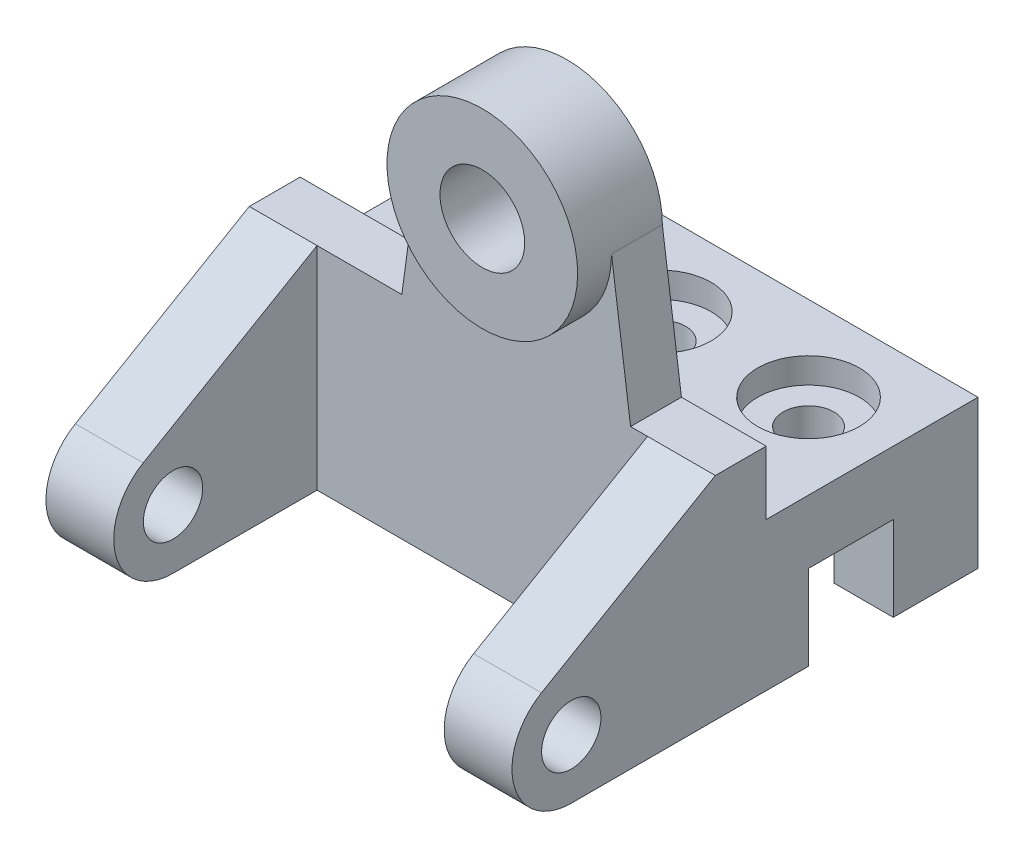
ISO-10303-21;
HEADER;
FILE_DESCRIPTION(('STEP AP214'),'2;1');
FILE_NAME('part.step','',(''),(''),'','','');
FILE_SCHEMA(('AUTOMOTIVE_DESIGN { 1 0 10303 214 1 1 1 1 }'));
ENDSEC;
DATA;
#1=APPLICATION_CONTEXT('core data for automotive mechanical design processes');
#2=APPLICATION_PROTOCOL_DEFINITION('international standard','automotive_design',2000,#1);
#3=PRODUCT_CONTEXT('',#1,'mechanical');
#4=PRODUCT('Part','Part','',(#3));
#5=PRODUCT_RELATED_PRODUCT_CATEGORY('part','',(#4));
#6=PRODUCT_DEFINITION_FORMATION('','',#4);
#7=PRODUCT_DEFINITION_CONTEXT('part definition',#1,'design');
#8=PRODUCT_DEFINITION('design','',#6,#7);
#9=PRODUCT_DEFINITION_SHAPE('','',#8);
#10=(LENGTH_UNIT() NAMED_UNIT(*) SI_UNIT(.MILLI.,.METRE.));
#11=(NAMED_UNIT(*) PLANE_ANGLE_UNIT() SI_UNIT($,.RADIAN.));
#12=(NAMED_UNIT(*) SI_UNIT($,.STERADIAN.) SOLID_ANGLE_UNIT());
#13=UNCERTAINTY_MEASURE_WITH_UNIT(LENGTH_MEASURE(1.E-05),#10,'distance_accuracy_value','');
#14=(GEOMETRIC_REPRESENTATION_CONTEXT(3) GLOBAL_UNCERTAINTY_ASSIGNED_CONTEXT((#13)) GLOBAL_UNIT_ASSIGNED_CONTEXT((#10,
#11,#12)) REPRESENTATION_CONTEXT('',''));
#15=CARTESIAN_POINT('',(0.,0.,0.));
#16=DIRECTION('',(0.,0.,1.));
#17=DIRECTION('',(1.,0.,0.));
#18=AXIS2_PLACEMENT_3D('',#15,#16,#17);
#19=CARTESIAN_POINT('',(-16.,0.,20.));
#20=DIRECTION('',(0.,0.,1.));
#21=DIRECTION('',(1.,0.,0.));
#22=AXIS2_PLACEMENT_3D('',#19,#20,#21);
#23=PLANE('',#22);
#24=DIRECTION('',(0.,1.,0.));
#25=VECTOR('',#24,1.);
#26=CARTESIAN_POINT('',(-14.,-28.999999999873,20.));
#27=LINE('',#26,#25);
#28=CARTESIAN_POINT('',(-14.,0.,20.));
#29=VERTEX_POINT('',#28);
#30=CARTESIAN_POINT('',(-14.,20.,20.));
#31=VERTEX_POINT('',#30);
#32=EDGE_CURVE('E54',#29,#31,#27,.T.);
#33=ORIENTED_EDGE('',*,*,#32,.F.);
#34=DIRECTION('',(1.,0.,0.));
#35=VECTOR('',#34,1.);
#36=CARTESIAN_POINT('',(-16.,0.,20.));
#37=LINE('',#36,#35);
#38=CARTESIAN_POINT('',(0.,0.,20.));
#39=VERTEX_POINT('',#38);
#40=EDGE_CURVE('E235',#29,#39,#37,.T.);
#41=ORIENTED_EDGE('',*,*,#40,.T.);
#42=DIRECTION('',(0.,-1.,0.));
#43=VECTOR('',#42,1.);
#44=CARTESIAN_POINT('',(0.,0.,20.));
#45=LINE('',#44,#43);
#46=CARTESIAN_POINT('',(0.,20.,20.));
#47=VERTEX_POINT('',#46);
#48=EDGE_CURVE('E443',#47,#39,#45,.T.);
#49=ORIENTED_EDGE('',*,*,#48,.F.);
#50=DIRECTION('',(1.,0.,0.));
#51=VECTOR('',#50,1.);
#52=CARTESIAN_POINT('',(-16.,20.,20.));
#53=LINE('',#52,#51);
#54=EDGE_CURVE('E237',#31,#47,#53,.T.);
#55=ORIENTED_EDGE('',*,*,#54,.F.);
#56=EDGE_LOOP('',(#33,#41,#49,#55));
#57=FACE_BOUND('',#56,.T.);
#58=ADVANCED_FACE('F41',(#57),#23,.T.);
#59=DIRECTION('',(0.,1.,0.));
#60=VECTOR('',#59,1.);
#61=CARTESIAN_POINT('',(-26.,-28.999999999873,20.));
#62=LINE('',#61,#60);
#63=CARTESIAN_POINT('',(-26.,20.,20.));
#64=VERTEX_POINT('',#63);
#65=CARTESIAN_POINT('',(-26.,0.,20.));
#66=VERTEX_POINT('',#65);
#67=EDGE_CURVE('E287',#64,#66,#62,.F.);
#68=ORIENTED_EDGE('',*,*,#67,.F.);
#69=CARTESIAN_POINT('',(-49.,20.,20.));
#70=VERTEX_POINT('',#69);
#71=EDGE_CURVE('E239',#70,#64,#53,.T.);
#72=ORIENTED_EDGE('',*,*,#71,.F.);
#73=DIRECTION('',(0.,1.,0.));
#74=VECTOR('',#73,1.);
#75=CARTESIAN_POINT('',(-49.,-28.999999999873,20.));
#76=LINE('',#75,#74);
#77=CARTESIAN_POINT('',(-49.,0.,20.));
#78=VERTEX_POINT('',#77);
#79=EDGE_CURVE('E61',#78,#70,#76,.T.);
#80=ORIENTED_EDGE('',*,*,#79,.F.);
#81=EDGE_CURVE('E240',#78,#66,#37,.T.);
#82=ORIENTED_EDGE('',*,*,#81,.T.);
#83=EDGE_LOOP('',(#68,#72,#80,#82));
#84=FACE_BOUND('',#83,.T.);
#85=ADVANCED_FACE('F453',(#84),#23,.T.);
#86=DIRECTION('',(0.,1.,0.));
#87=VECTOR('',#86,1.);
#88=CARTESIAN_POINT('',(-61.,-28.999999999873,20.));
#89=LINE('',#88,#87);
#90=CARTESIAN_POINT('',(-61.,20.,20.));
#91=VERTEX_POINT('',#90);
#92=CARTESIAN_POINT('',(-61.,0.,20.));
#93=VERTEX_POINT('',#92);
#94=EDGE_CURVE('E273',#91,#93,#89,.F.);
#95=ORIENTED_EDGE('',*,*,#94,.F.);
#96=CARTESIAN_POINT('',(-84.,20.,20.));
#97=VERTEX_POINT('',#96);
#98=EDGE_CURVE('E233',#97,#91,#53,.T.);
#99=ORIENTED_EDGE('',*,*,#98,.F.);
#100=DIRECTION('',(0.,1.,0.));
#101=VECTOR('',#100,1.);
#102=CARTESIAN_POINT('',(-84.,-28.999999999873,20.));
#103=LINE('',#102,#101);
#104=CARTESIAN_POINT('',(-84.,0.,20.));
#105=VERTEX_POINT('',#104);
#106=EDGE_CURVE('E213',#105,#97,#103,.T.);
#107=ORIENTED_EDGE('',*,*,#106,.F.);
#108=EDGE_CURVE('E283',#105,#93,#37,.T.);
#109=ORIENTED_EDGE('',*,*,#108,.T.);
#110=EDGE_LOOP('',(#95,#99,#107,#109));
#111=FACE_BOUND('',#110,.T.);
#112=ADVANCED_FACE('F276',(#111),#23,.T.);
#113=CARTESIAN_POINT('',(-16.,50.000000000127,50.000000000074));
#114=DIRECTION('',(0.,1.,0.));
#115=DIRECTION('',(0.,0.,1.));
#116=AXIS2_PLACEMENT_3D('',#113,#114,#115);
#117=PLANE('',#116);
#118=DIRECTION('',(1.,0.,0.));
#119=VECTOR('',#118,1.);
#120=CARTESIAN_POINT('',(-16.,50.000000000127,50.000000000074));
#121=LINE('',#120,#119);
#122=CARTESIAN_POINT('',(-20.,50.000000000127,50.000000000074));
#123=VERTEX_POINT('',#122);
#124=CARTESIAN_POINT('',(0.,50.000000000127,50.000000000074));
#125=VERTEX_POINT('',#124);
#126=EDGE_CURVE('E261',#123,#125,#121,.T.);
#127=ORIENTED_EDGE('',*,*,#126,.F.);
#128=DIRECTION('',(0.,0.,1.));
#129=VECTOR('',#128,1.);
#130=CARTESIAN_POINT('',(-20.,50.000000000127,50.000000000074));
#131=LINE('',#130,#129);
#132=CARTESIAN_POINT('',(-20.,50.000000000127,62.000000000074));
#133=VERTEX_POINT('',#132);
#134=EDGE_CURVE('E332',#123,#133,#131,.T.);
#135=ORIENTED_EDGE('',*,*,#134,.T.);
#136=DIRECTION('',(1.,0.,0.));
#137=VECTOR('',#136,1.);
#138=CARTESIAN_POINT('',(-110.,50.000000000127,62.000000000074));
#139=LINE('',#138,#137);
#140=CARTESIAN_POINT('',(-16.,50.000000000127,62.000000000074));
#141=VERTEX_POINT('',#140);
#142=EDGE_CURVE('E397',#133,#141,#139,.T.);
#143=ORIENTED_EDGE('',*,*,#142,.T.);
#144=DIRECTION('',(1.,0.,0.));
#145=VECTOR('',#144,1.);
#146=CARTESIAN_POINT('',(-16.,50.000000000127,62.000000000074));
#147=LINE('',#146,#145);
#148=CARTESIAN_POINT('',(0.,50.000000000127,62.000000000074));
#149=VERTEX_POINT('',#148);
#150=EDGE_CURVE('E258',#141,#149,#147,.T.);
#151=ORIENTED_EDGE('',*,*,#150,.T.);
#152=DIRECTION('',(0.,0.,1.));
#153=VECTOR('',#152,1.);
#154=CARTESIAN_POINT('',(0.,50.000000000127,50.000000000074));
#155=LINE('',#154,#153);
#156=EDGE_CURVE('E430',#125,#149,#155,.T.);
#157=ORIENTED_EDGE('',*,*,#156,.F.);
#158=EDGE_LOOP('',(#127,#135,#143,#151,#157));
#159=FACE_BOUND('',#158,.T.);
#160=ADVANCED_FACE('F559',(#159),#117,.T.);
#161=CARTESIAN_POINT('',(-110.,50.000000000127,62.000000000074));
#162=DIRECTION('',(0.,0.,-1.));
#163=DIRECTION('',(-1.,0.,0.));
#164=AXIS2_PLACEMENT_3D('',#161,#162,#163);
#165=PLANE('',#164);
#166=DIRECTION('',(0.,-1.,0.));
#167=VECTOR('',#166,1.);
#168=CARTESIAN_POINT('',(-94.,0.,62.000000000074));
#169=LINE('',#168,#167);
#170=CARTESIAN_POINT('',(-94.,50.000000000127,62.000000000074));
#171=VERTEX_POINT('',#170);
#172=CARTESIAN_POINT('',(-94.,0.,62.000000000074));
#173=VERTEX_POINT('',#172);
#174=EDGE_CURVE('E364',#171,#173,#169,.T.);
#175=ORIENTED_EDGE('',*,*,#174,.T.);
#176=DIRECTION('',(1.,0.,0.));
#177=VECTOR('',#176,1.);
#178=CARTESIAN_POINT('',(-110.,0.,62.000000000074));
#179=LINE('',#178,#177);
#180=CARTESIAN_POINT('',(-16.,0.,62.000000000074));
#181=VERTEX_POINT('',#180);
#182=EDGE_CURVE('E408',#173,#181,#179,.T.);
#183=ORIENTED_EDGE('',*,*,#182,.T.);
#184=DIRECTION('',(0.,1.,0.));
#185=VECTOR('',#184,1.);
#186=CARTESIAN_POINT('',(-16.,50.000000000127,62.000000000074));
#187=LINE('',#186,#185);
#188=EDGE_CURVE('E372',#181,#141,#187,.T.);
#189=ORIENTED_EDGE('',*,*,#188,.T.);
#190=ORIENTED_EDGE('',*,*,#142,.F.);
#191=DIRECTION('',(-0.135113204733824,0.990830168044229,0.));
#192=VECTOR('',#191,1.);
#193=CARTESIAN_POINT('',(-20.,50.000000000127,62.000000000074));
#194=LINE('',#193,#192);
#195=CARTESIAN_POINT('',(-24.5,83.,62.000000000074));
#196=VERTEX_POINT('',#195);
#197=EDGE_CURVE('E322',#133,#196,#194,.T.);
#198=ORIENTED_EDGE('',*,*,#197,.T.);
#199=CARTESIAN_POINT('',(-47.,83.,62.000000000074));
#200=DIRECTION('',(0.,0.,-1.));
#201=DIRECTION('',(1.,0.,0.));
#202=AXIS2_PLACEMENT_3D('',#199,#200,#201);
#203=CIRCLE('',#202,22.5);
#204=CARTESIAN_POINT('',(-69.5,83.,62.000000000074));
#205=VERTEX_POINT('',#204);
#206=EDGE_CURVE('E331',#196,#205,#203,.T.);
#207=ORIENTED_EDGE('',*,*,#206,.T.);
#208=DIRECTION('',(-0.135113204733824,-0.990830168044229,0.));
#209=VECTOR('',#208,1.);
#210=CARTESIAN_POINT('',(-74.,50.000000000127,62.000000000074));
#211=LINE('',#210,#209);
#212=CARTESIAN_POINT('',(-74.,50.000000000127,62.000000000074));
#213=VERTEX_POINT('',#212);
#214=EDGE_CURVE('E328',#205,#213,#211,.T.);
#215=ORIENTED_EDGE('',*,*,#214,.T.);
#216=EDGE_CURVE('E410',#171,#213,#139,.T.);
#217=ORIENTED_EDGE('',*,*,#216,.F.);
#218=EDGE_LOOP('',(#175,#183,#189,#190,#198,#207,#215,#217));
#219=FACE_BOUND('',#218,.T.);
#220=ADVANCED_FACE('F563',(#219),#165,.F.);
#221=CARTESIAN_POINT('',(-16.,14.,96.));
#222=DIRECTION('',(1.,0.,0.));
#223=DIRECTION('',(0.,0.,-1.));
#224=AXIS2_PLACEMENT_3D('',#221,#222,#223);
#225=PLANE('',#224);
#226=CARTESIAN_POINT('',(-16.,14.,96.));
#227=DIRECTION('',(1.,0.,0.));
#228=DIRECTION('',(0.,0.,-1.));
#229=AXIS2_PLACEMENT_3D('',#226,#227,#228);
#230=CIRCLE('',#229,7.);
#231=CARTESIAN_POINT('',(-16.,14.,89.));
#232=VERTEX_POINT('',#231);
#233=EDGE_CURVE('E355',#232,#232,#230,.T.);
#234=ORIENTED_EDGE('',*,*,#233,.T.);
#235=EDGE_LOOP('',(#234));
#236=FACE_BOUND('',#235,.T.);
#237=ORIENTED_EDGE('',*,*,#188,.F.);
#238=DIRECTION('',(0.,0.,-1.));
#239=VECTOR('',#238,1.);
#240=CARTESIAN_POINT('',(-16.,0.,40.));
#241=LINE('',#240,#239);
#242=CARTESIAN_POINT('',(-16.,0.,96.));
#243=VERTEX_POINT('',#242);
#244=EDGE_CURVE('E266',#243,#181,#241,.T.);
#245=ORIENTED_EDGE('',*,*,#244,.F.);
#246=CARTESIAN_POINT('',(-16.,14.,96.));
#247=DIRECTION('',(1.,0.,0.));
#248=DIRECTION('',(0.,0.,-1.));
#249=AXIS2_PLACEMENT_3D('',#246,#247,#248);
#250=CIRCLE('',#249,14.);
#251=CARTESIAN_POINT('',(-16.,26.0981840675639,103.045136071599));
#252=VERTEX_POINT('',#251);
#253=EDGE_CURVE('E415',#252,#243,#250,.T.);
#254=ORIENTED_EDGE('',*,*,#253,.F.);
#255=DIRECTION('',(0.,-0.5032240051142,0.864156004825994));
#256=VECTOR('',#255,1.);
#257=CARTESIAN_POINT('',(-16.,50.000000000127,62.000000000074));
#258=LINE('',#257,#256);
#259=EDGE_CURVE('E409',#141,#252,#258,.T.);
#260=ORIENTED_EDGE('',*,*,#259,.F.);
#261=EDGE_LOOP('',(#237,#245,#254,#260));
#262=FACE_BOUND('',#261,.T.);
#263=ADVANCED_FACE('F573',(#236,#262),#225,.F.);
#264=CARTESIAN_POINT('',(-16.,0.,0.));
#265=DIRECTION('',(0.,0.,-1.));
#266=DIRECTION('',(0.,1.,0.));
#267=AXIS2_PLACEMENT_3D('',#264,#265,#266);
#268=PLANE('',#267);
#269=DIRECTION('',(0.,1.,0.));
#270=VECTOR('',#269,1.);
#271=CARTESIAN_POINT('',(0.,0.,0.));
#272=LINE('',#271,#270);
#273=CARTESIAN_POINT('',(0.,0.,0.));
#274=VERTEX_POINT('',#273);
#275=CARTESIAN_POINT('',(0.,35.0000000001271,0.));
#276=VERTEX_POINT('',#275);
#277=EDGE_CURVE('E407',#274,#276,#272,.T.);
#278=ORIENTED_EDGE('',*,*,#277,.F.);
#279=DIRECTION('',(1.,0.,0.));
#280=VECTOR('',#279,1.);
#281=CARTESIAN_POINT('',(-16.,0.,0.));
#282=LINE('',#281,#280);
#283=CARTESIAN_POINT('',(-110.,0.,0.));
#284=VERTEX_POINT('',#283);
#285=EDGE_CURVE('E217',#284,#274,#282,.T.);
#286=ORIENTED_EDGE('',*,*,#285,.F.);
#287=DIRECTION('',(0.,-1.,0.));
#288=VECTOR('',#287,1.);
#289=CARTESIAN_POINT('',(-110.,0.,0.));
#290=LINE('',#289,#288);
#291=CARTESIAN_POINT('',(-110.,35.0000000001271,0.));
#292=VERTEX_POINT('',#291);
#293=EDGE_CURVE('E396',#292,#284,#290,.T.);
#294=ORIENTED_EDGE('',*,*,#293,.F.);
#295=DIRECTION('',(1.,0.,0.));
#296=VECTOR('',#295,1.);
#297=CARTESIAN_POINT('',(-16.,35.0000000001271,0.));
#298=LINE('',#297,#296);
#299=EDGE_CURVE('E262',#292,#276,#298,.T.);
#300=ORIENTED_EDGE('',*,*,#299,.T.);
#301=EDGE_LOOP('',(#278,#286,#294,#300));
#302=FACE_BOUND('',#301,.T.);
#303=ADVANCED_FACE('F43',(#302),#268,.T.);
#304=CARTESIAN_POINT('',(-16.,0.,0.));
#305=DIRECTION('',(0.,-1.,0.));
#306=DIRECTION('',(0.,0.,-1.));
#307=AXIS2_PLACEMENT_3D('',#304,#305,#306);
#308=PLANE('',#307);
#309=CARTESIAN_POINT('',(-20.,0.,20.000000000074));
#310=DIRECTION('',(0.,-1.,0.));
#311=DIRECTION('',(0.,0.,-1.));
#312=AXIS2_PLACEMENT_3D('',#309,#310,#311);
#313=CIRCLE('',#312,6.);
#314=EDGE_CURVE('E291',#66,#29,#313,.T.);
#315=ORIENTED_EDGE('',*,*,#314,.F.);
#316=ORIENTED_EDGE('',*,*,#81,.F.);
#317=CARTESIAN_POINT('',(-55.,0.,20.000000000074));
#318=DIRECTION('',(0.,-1.,0.));
#319=DIRECTION('',(0.,0.,-1.));
#320=AXIS2_PLACEMENT_3D('',#317,#318,#319);
#321=CIRCLE('',#320,6.);
#322=EDGE_CURVE('E282',#93,#78,#321,.T.);
#323=ORIENTED_EDGE('',*,*,#322,.F.);
#324=ORIENTED_EDGE('',*,*,#108,.F.);
#325=CARTESIAN_POINT('',(-90.,0.,20.000000000074));
#326=DIRECTION('',(0.,-1.,0.));
#327=DIRECTION('',(0.,0.,-1.));
#328=AXIS2_PLACEMENT_3D('',#325,#326,#327);
#329=CIRCLE('',#328,6.);
#330=CARTESIAN_POINT('',(-96.,0.,20.));
#331=VERTEX_POINT('',#330);
#332=EDGE_CURVE('E285',#331,#105,#329,.T.);
#333=ORIENTED_EDGE('',*,*,#332,.F.);
#334=CARTESIAN_POINT('',(-110.,0.,20.));
#335=VERTEX_POINT('',#334);
#336=EDGE_CURVE('E228',#335,#331,#37,.T.);
#337=ORIENTED_EDGE('',*,*,#336,.F.);
#338=DIRECTION('',(0.,0.,1.));
#339=VECTOR('',#338,1.);
#340=CARTESIAN_POINT('',(-110.,0.,20.));
#341=LINE('',#340,#339);
#342=EDGE_CURVE('E380',#284,#335,#341,.T.);
#343=ORIENTED_EDGE('',*,*,#342,.F.);
#344=ORIENTED_EDGE('',*,*,#285,.T.);
#345=DIRECTION('',(0.,0.,-1.));
#346=VECTOR('',#345,1.);
#347=CARTESIAN_POINT('',(0.,0.,0.));
#348=LINE('',#347,#346);
#349=EDGE_CURVE('E413',#39,#274,#348,.T.);
#350=ORIENTED_EDGE('',*,*,#349,.F.);
#351=ORIENTED_EDGE('',*,*,#40,.F.);
#352=EDGE_LOOP('',(#315,#316,#323,#324,#333,#337,#343,#344,#350,#351));
#353=FACE_BOUND('',#352,.T.);
#354=ADVANCED_FACE('F460',(#353),#308,.T.);
#355=DIRECTION('',(0.,1.,0.));
#356=VECTOR('',#355,1.);
#357=CARTESIAN_POINT('',(-96.,-28.999999999873,20.));
#358=LINE('',#357,#356);
#359=CARTESIAN_POINT('',(-96.,20.,20.));
#360=VERTEX_POINT('',#359);
#361=EDGE_CURVE('E209',#360,#331,#358,.F.);
#362=ORIENTED_EDGE('',*,*,#361,.F.);
#363=CARTESIAN_POINT('',(-110.,20.,20.));
#364=VERTEX_POINT('',#363);
#365=EDGE_CURVE('E221',#364,#360,#53,.T.);
#366=ORIENTED_EDGE('',*,*,#365,.F.);
#367=DIRECTION('',(0.,1.,0.));
#368=VECTOR('',#367,1.);
#369=CARTESIAN_POINT('',(-110.,20.,20.));
#370=LINE('',#369,#368);
#371=EDGE_CURVE('E379',#335,#364,#370,.T.);
#372=ORIENTED_EDGE('',*,*,#371,.F.);
#373=ORIENTED_EDGE('',*,*,#336,.T.);
#374=EDGE_LOOP('',(#362,#366,#372,#373));
#375=FACE_BOUND('',#374,.T.);
#376=ADVANCED_FACE('F225',(#375),#23,.T.);
#377=CARTESIAN_POINT('',(-16.,20.,20.));
#378=DIRECTION('',(0.,-1.,0.));
#379=DIRECTION('',(0.,0.,-1.));
#380=AXIS2_PLACEMENT_3D('',#377,#378,#379);
#381=PLANE('',#380);
#382=CARTESIAN_POINT('',(-20.,20.,20.000000000074));
#383=DIRECTION('',(0.,-1.,0.));
#384=DIRECTION('',(0.,0.,-1.));
#385=AXIS2_PLACEMENT_3D('',#382,#383,#384);
#386=CIRCLE('',#385,6.);
#387=EDGE_CURVE('E11',#31,#64,#386,.T.);
#388=ORIENTED_EDGE('',*,*,#387,.F.);
#389=ORIENTED_EDGE('',*,*,#54,.T.);
#390=DIRECTION('',(0.,0.,-1.));
#391=VECTOR('',#390,1.);
#392=CARTESIAN_POINT('',(0.,20.,20.));
#393=LINE('',#392,#391);
#394=CARTESIAN_POINT('',(0.,20.,40.));
#395=VERTEX_POINT('',#394);
#396=EDGE_CURVE('E445',#395,#47,#393,.T.);
#397=ORIENTED_EDGE('',*,*,#396,.F.);
#398=DIRECTION('',(1.,0.,0.));
#399=VECTOR('',#398,1.);
#400=CARTESIAN_POINT('',(-16.,20.,40.));
#401=LINE('',#400,#399);
#402=CARTESIAN_POINT('',(-110.,20.,40.));
#403=VERTEX_POINT('',#402);
#404=EDGE_CURVE('E243',#403,#395,#401,.T.);
#405=ORIENTED_EDGE('',*,*,#404,.F.);
#406=DIRECTION('',(0.,0.,1.));
#407=VECTOR('',#406,1.);
#408=CARTESIAN_POINT('',(-110.,20.,40.));
#409=LINE('',#408,#407);
#410=EDGE_CURVE('E231',#364,#403,#409,.T.);
#411=ORIENTED_EDGE('',*,*,#410,.F.);
#412=ORIENTED_EDGE('',*,*,#365,.T.);
#413=CARTESIAN_POINT('',(-90.,20.,20.000000000074));
#414=DIRECTION('',(0.,-1.,0.));
#415=DIRECTION('',(0.,0.,-1.));
#416=AXIS2_PLACEMENT_3D('',#413,#414,#415);
#417=CIRCLE('',#416,6.);
#418=EDGE_CURVE('E206',#97,#360,#417,.T.);
#419=ORIENTED_EDGE('',*,*,#418,.F.);
#420=ORIENTED_EDGE('',*,*,#98,.T.);
#421=CARTESIAN_POINT('',(-55.,20.,20.000000000074));
#422=DIRECTION('',(0.,-1.,0.));
#423=DIRECTION('',(0.,0.,-1.));
#424=AXIS2_PLACEMENT_3D('',#421,#422,#423);
#425=CIRCLE('',#424,6.);
#426=EDGE_CURVE('E47',#70,#91,#425,.T.);
#427=ORIENTED_EDGE('',*,*,#426,.F.);
#428=ORIENTED_EDGE('',*,*,#71,.T.);
#429=EDGE_LOOP('',(#388,#389,#397,#405,#411,#412,#419,#420,#427,#428));
#430=FACE_BOUND('',#429,.T.);
#431=ADVANCED_FACE('F229',(#430),#381,.T.);
#432=CARTESIAN_POINT('',(-16.,20.,40.));
#433=DIRECTION('',(0.,0.,-1.));
#434=DIRECTION('',(-1.,0.,0.));
#435=AXIS2_PLACEMENT_3D('',#432,#433,#434);
#436=PLANE('',#435);
#437=DIRECTION('',(0.,1.,0.));
#438=VECTOR('',#437,1.);
#439=CARTESIAN_POINT('',(0.,20.,40.));
#440=LINE('',#439,#438);
#441=CARTESIAN_POINT('',(0.,0.,40.));
#442=VERTEX_POINT('',#441);
#443=EDGE_CURVE('E438',#442,#395,#440,.T.);
#444=ORIENTED_EDGE('',*,*,#443,.F.);
#445=DIRECTION('',(1.,0.,0.));
#446=VECTOR('',#445,1.);
#447=CARTESIAN_POINT('',(-16.,0.,40.));
#448=LINE('',#447,#446);
#449=CARTESIAN_POINT('',(-110.,0.,40.));
#450=VERTEX_POINT('',#449);
#451=EDGE_CURVE('E249',#450,#442,#448,.T.);
#452=ORIENTED_EDGE('',*,*,#451,.F.);
#453=DIRECTION('',(0.,-1.,0.));
#454=VECTOR('',#453,1.);
#455=CARTESIAN_POINT('',(-110.,0.,40.));
#456=LINE('',#455,#454);
#457=EDGE_CURVE('E382',#403,#450,#456,.T.);
#458=ORIENTED_EDGE('',*,*,#457,.F.);
#459=ORIENTED_EDGE('',*,*,#404,.T.);
#460=EDGE_LOOP('',(#444,#452,#458,#459));
#461=FACE_BOUND('',#460,.T.);
#462=ADVANCED_FACE('F470',(#461),#436,.T.);
#463=CARTESIAN_POINT('',(-16.,0.,40.));
#464=DIRECTION('',(0.,-1.,0.));
#465=DIRECTION('',(0.,0.,-1.));
#466=AXIS2_PLACEMENT_3D('',#463,#464,#465);
#467=PLANE('',#466);
#468=DIRECTION('',(0.,0.,-1.));
#469=VECTOR('',#468,1.);
#470=CARTESIAN_POINT('',(0.,0.,40.));
#471=LINE('',#470,#469);
#472=CARTESIAN_POINT('',(0.,0.,96.));
#473=VERTEX_POINT('',#472);
#474=EDGE_CURVE('E436',#473,#442,#471,.T.);
#475=ORIENTED_EDGE('',*,*,#474,.F.);
#476=DIRECTION('',(1.,0.,0.));
#477=VECTOR('',#476,1.);
#478=CARTESIAN_POINT('',(-16.,0.,96.));
#479=LINE('',#478,#477);
#480=EDGE_CURVE('E247',#243,#473,#479,.T.);
#481=ORIENTED_EDGE('',*,*,#480,.F.);
#482=ORIENTED_EDGE('',*,*,#244,.T.);
#483=ORIENTED_EDGE('',*,*,#182,.F.);
#484=DIRECTION('',(0.,0.,1.));
#485=VECTOR('',#484,1.);
#486=CARTESIAN_POINT('',(-94.,0.,62.000000000074));
#487=LINE('',#486,#485);
#488=CARTESIAN_POINT('',(-94.,0.,96.0000000000002));
#489=VERTEX_POINT('',#488);
#490=EDGE_CURVE('E359',#173,#489,#487,.T.);
#491=ORIENTED_EDGE('',*,*,#490,.T.);
#492=DIRECTION('',(-1.,0.,0.));
#493=VECTOR('',#492,1.);
#494=CARTESIAN_POINT('',(-94.,0.,96.0000000000002));
#495=LINE('',#494,#493);
#496=CARTESIAN_POINT('',(-110.,0.,96.0000000000002));
#497=VERTEX_POINT('',#496);
#498=EDGE_CURVE('E366',#489,#497,#495,.T.);
#499=ORIENTED_EDGE('',*,*,#498,.T.);
#500=DIRECTION('',(0.,0.,1.));
#501=VECTOR('',#500,1.);
#502=CARTESIAN_POINT('',(-110.,0.,62.000000000074));
#503=LINE('',#502,#501);
#504=EDGE_CURVE('E387',#450,#497,#503,.T.);
#505=ORIENTED_EDGE('',*,*,#504,.F.);
#506=ORIENTED_EDGE('',*,*,#451,.T.);
#507=EDGE_LOOP('',(#475,#481,#482,#483,#491,#499,#505,#506));
#508=FACE_BOUND('',#507,.T.);
#509=ADVANCED_FACE('F473',(#508),#467,.T.);
#510=CARTESIAN_POINT('',(-16.,14.,96.));
#511=DIRECTION('',(1.,0.,0.));
#512=DIRECTION('',(0.,0.,-1.));
#513=AXIS2_PLACEMENT_3D('',#510,#511,#512);
#514=CYLINDRICAL_SURFACE('',#513,14.);
#515=CARTESIAN_POINT('',(0.,14.,96.));
#516=DIRECTION('',(1.,0.,0.));
#517=DIRECTION('',(0.,0.,-1.));
#518=AXIS2_PLACEMENT_3D('',#515,#516,#517);
#519=CIRCLE('',#518,14.);
#520=CARTESIAN_POINT('',(0.,26.0981840675639,103.045136071599));
#521=VERTEX_POINT('',#520);
#522=EDGE_CURVE('E433',#521,#473,#519,.T.);
#523=ORIENTED_EDGE('',*,*,#522,.F.);
#524=DIRECTION('',(1.,0.,0.));
#525=VECTOR('',#524,1.);
#526=CARTESIAN_POINT('',(-16.,26.0981840675639,103.045136071599));
#527=LINE('',#526,#525);
#528=EDGE_CURVE('E255',#252,#521,#527,.T.);
#529=ORIENTED_EDGE('',*,*,#528,.F.);
#530=ORIENTED_EDGE('',*,*,#253,.T.);
#531=ORIENTED_EDGE('',*,*,#480,.T.);
#532=EDGE_LOOP('',(#523,#529,#530,#531));
#533=FACE_BOUND('',#532,.T.);
#534=ADVANCED_FACE('F584',(#533),#514,.T.);
#535=CARTESIAN_POINT('',(-16.,50.000000000127,62.000000000074));
#536=DIRECTION('',(0.,0.864156004825994,0.5032240051142));
#537=DIRECTION('',(0.,-0.5032240051142,0.864156004825994));
#538=AXIS2_PLACEMENT_3D('',#535,#536,#537);
#539=PLANE('',#538);
#540=DIRECTION('',(0.,-0.5032240051142,0.864156004825994));
#541=VECTOR('',#540,1.);
#542=CARTESIAN_POINT('',(0.,50.000000000127,62.000000000074));
#543=LINE('',#542,#541);
#544=EDGE_CURVE('E429',#149,#521,#543,.T.);
#545=ORIENTED_EDGE('',*,*,#544,.F.);
#546=ORIENTED_EDGE('',*,*,#150,.F.);
#547=ORIENTED_EDGE('',*,*,#259,.T.);
#548=ORIENTED_EDGE('',*,*,#528,.T.);
#549=EDGE_LOOP('',(#545,#546,#547,#548));
#550=FACE_BOUND('',#549,.T.);
#551=ADVANCED_FACE('F580',(#550),#539,.T.);
#552=DIRECTION('',(0.,0.,1.));
#553=VECTOR('',#552,1.);
#554=CARTESIAN_POINT('',(-74.,50.000000000127,50.000000000074));
#555=LINE('',#554,#553);
#556=CARTESIAN_POINT('',(-74.,50.000000000127,50.000000000074));
#557=VERTEX_POINT('',#556);
#558=EDGE_CURVE('E337',#557,#213,#555,.T.);
#559=ORIENTED_EDGE('',*,*,#558,.F.);
#560=CARTESIAN_POINT('',(-110.,50.000000000127,50.000000000074));
#561=VERTEX_POINT('',#560);
#562=EDGE_CURVE('E256',#561,#557,#121,.T.);
#563=ORIENTED_EDGE('',*,*,#562,.F.);
#564=DIRECTION('',(0.,0.,-1.));
#565=VECTOR('',#564,1.);
#566=CARTESIAN_POINT('',(-110.,50.000000000127,50.000000000074));
#567=LINE('',#566,#565);
#568=CARTESIAN_POINT('',(-110.,50.000000000127,62.000000000074));
#569=VERTEX_POINT('',#568);
#570=EDGE_CURVE('E389',#569,#561,#567,.T.);
#571=ORIENTED_EDGE('',*,*,#570,.F.);
#572=EDGE_CURVE('E401',#569,#171,#139,.T.);
#573=ORIENTED_EDGE('',*,*,#572,.T.);
#574=ORIENTED_EDGE('',*,*,#216,.T.);
#575=EDGE_LOOP('',(#559,#563,#571,#573,#574));
#576=FACE_BOUND('',#575,.T.);
#577=ADVANCED_FACE('F486',(#576),#117,.T.);
#578=CARTESIAN_POINT('',(-16.,35.0000000001271,50.000000000074));
#579=DIRECTION('',(0.,0.,-1.));
#580=DIRECTION('',(0.,1.,0.));
#581=AXIS2_PLACEMENT_3D('',#578,#579,#580);
#582=PLANE('',#581);
#583=CARTESIAN_POINT('',(-47.,83.,50.000000000074));
#584=DIRECTION('',(0.,0.,-1.));
#585=DIRECTION('',(0.,1.,0.));
#586=AXIS2_PLACEMENT_3D('',#583,#584,#585);
#587=CIRCLE('',#586,10.);
#588=CARTESIAN_POINT('',(-47.,93.,50.000000000074));
#589=VERTEX_POINT('',#588);
#590=EDGE_CURVE('E316',#589,#589,#587,.T.);
#591=ORIENTED_EDGE('',*,*,#590,.F.);
#592=EDGE_LOOP('',(#591));
#593=FACE_BOUND('',#592,.T.);
#594=DIRECTION('',(0.,1.,0.));
#595=VECTOR('',#594,1.);
#596=CARTESIAN_POINT('',(0.,35.0000000001271,50.000000000074));
#597=LINE('',#596,#595);
#598=CARTESIAN_POINT('',(0.,35.0000000001271,50.000000000074));
#599=VERTEX_POINT('',#598);
#600=EDGE_CURVE('E424',#599,#125,#597,.T.);
#601=ORIENTED_EDGE('',*,*,#600,.F.);
#602=DIRECTION('',(1.,0.,0.));
#603=VECTOR('',#602,1.);
#604=CARTESIAN_POINT('',(-16.,35.0000000001271,50.000000000074));
#605=LINE('',#604,#603);
#606=CARTESIAN_POINT('',(-110.,35.0000000001271,50.000000000074));
#607=VERTEX_POINT('',#606);
#608=EDGE_CURVE('E265',#607,#599,#605,.T.);
#609=ORIENTED_EDGE('',*,*,#608,.F.);
#610=DIRECTION('',(0.,-1.,0.));
#611=VECTOR('',#610,1.);
#612=CARTESIAN_POINT('',(-110.,35.0000000001271,50.000000000074));
#613=LINE('',#612,#611);
#614=EDGE_CURVE('E393',#561,#607,#613,.T.);
#615=ORIENTED_EDGE('',*,*,#614,.F.);
#616=ORIENTED_EDGE('',*,*,#562,.T.);
#617=DIRECTION('',(-0.135113204733824,-0.990830168044229,0.));
#618=VECTOR('',#617,1.);
#619=CARTESIAN_POINT('',(-74.,50.000000000127,50.000000000074));
#620=LINE('',#619,#618);
#621=CARTESIAN_POINT('',(-69.5,83.,50.000000000074));
#622=VERTEX_POINT('',#621);
#623=EDGE_CURVE('E327',#622,#557,#620,.T.);
#624=ORIENTED_EDGE('',*,*,#623,.F.);
#625=CARTESIAN_POINT('',(-47.,83.,50.000000000074));
#626=DIRECTION('',(0.,0.,1.));
#627=DIRECTION('',(1.,0.,0.));
#628=AXIS2_PLACEMENT_3D('',#625,#626,#627);
#629=CIRCLE('',#628,22.5);
#630=CARTESIAN_POINT('',(-24.5,83.,50.000000000074));
#631=VERTEX_POINT('',#630);
#632=EDGE_CURVE('E325',#631,#622,#629,.T.);
#633=ORIENTED_EDGE('',*,*,#632,.F.);
#634=DIRECTION('',(-0.135113204733824,0.990830168044229,0.));
#635=VECTOR('',#634,1.);
#636=CARTESIAN_POINT('',(-20.,50.000000000127,50.000000000074));
#637=LINE('',#636,#635);
#638=EDGE_CURVE('E324',#123,#631,#637,.T.);
#639=ORIENTED_EDGE('',*,*,#638,.F.);
#640=ORIENTED_EDGE('',*,*,#126,.T.);
#641=EDGE_LOOP('',(#601,#609,#615,#616,#624,#633,#639,#640));
#642=FACE_BOUND('',#641,.T.);
#643=ADVANCED_FACE('F491',(#593,#642),#582,.T.);
#644=CARTESIAN_POINT('',(-16.,35.0000000001271,0.));
#645=DIRECTION('',(0.,1.,0.));
#646=DIRECTION('',(0.,0.,1.));
#647=AXIS2_PLACEMENT_3D('',#644,#645,#646);
#648=PLANE('',#647);
#649=CARTESIAN_POINT('',(-20.,35.0000000001271,20.000000000074));
#650=DIRECTION('',(0.,1.,0.));
#651=DIRECTION('',(0.,0.,1.));
#652=AXIS2_PLACEMENT_3D('',#649,#650,#651);
#653=CIRCLE('',#652,12.);
#654=CARTESIAN_POINT('',(-20.,35.0000000001271,32.000000000074));
#655=VERTEX_POINT('',#654);
#656=EDGE_CURVE('E299',#655,#655,#653,.T.);
#657=ORIENTED_EDGE('',*,*,#656,.F.);
#658=EDGE_LOOP('',(#657));
#659=FACE_BOUND('',#658,.T.);
#660=CARTESIAN_POINT('',(-55.,35.0000000001271,20.000000000074));
#661=DIRECTION('',(0.,1.,0.));
#662=DIRECTION('',(0.,0.,1.));
#663=AXIS2_PLACEMENT_3D('',#660,#661,#662);
#664=CIRCLE('',#663,12.);
#665=CARTESIAN_POINT('',(-55.,35.0000000001271,32.000000000074));
#666=VERTEX_POINT('',#665);
#667=EDGE_CURVE('E308',#666,#666,#664,.T.);
#668=ORIENTED_EDGE('',*,*,#667,.F.);
#669=EDGE_LOOP('',(#668));
#670=FACE_BOUND('',#669,.T.);
#671=CARTESIAN_POINT('',(-90.,35.0000000001271,20.000000000074));
#672=DIRECTION('',(0.,1.,0.));
#673=DIRECTION('',(0.,0.,1.));
#674=AXIS2_PLACEMENT_3D('',#671,#672,#673);
#675=CIRCLE('',#674,12.0000000000216);
#676=CARTESIAN_POINT('',(-90.,35.0000000001271,32.0000000000956));
#677=VERTEX_POINT('',#676);
#678=EDGE_CURVE('E293',#677,#677,#675,.T.);
#679=ORIENTED_EDGE('',*,*,#678,.F.);
#680=EDGE_LOOP('',(#679));
#681=FACE_BOUND('',#680,.T.);
#682=DIRECTION('',(0.,0.,1.));
#683=VECTOR('',#682,1.);
#684=CARTESIAN_POINT('',(0.,35.0000000001271,0.));
#685=LINE('',#684,#683);
#686=EDGE_CURVE('E423',#276,#599,#685,.T.);
#687=ORIENTED_EDGE('',*,*,#686,.F.);
#688=ORIENTED_EDGE('',*,*,#299,.F.);
#689=DIRECTION('',(0.,0.,-1.));
#690=VECTOR('',#689,1.);
#691=CARTESIAN_POINT('',(-110.,35.0000000001271,0.));
#692=LINE('',#691,#690);
#693=EDGE_CURVE('E392',#607,#292,#692,.T.);
#694=ORIENTED_EDGE('',*,*,#693,.F.);
#695=ORIENTED_EDGE('',*,*,#608,.T.);
#696=EDGE_LOOP('',(#687,#688,#694,#695));
#697=FACE_BOUND('',#696,.T.);
#698=ADVANCED_FACE('F494',(#659,#670,#681,#697),#648,.T.);
#699=CARTESIAN_POINT('',(0.,14.,96.));
#700=DIRECTION('',(1.,0.,0.));
#701=DIRECTION('',(0.,0.,-1.));
#702=AXIS2_PLACEMENT_3D('',#699,#700,#701);
#703=PLANE('',#702);
#704=CARTESIAN_POINT('',(0.,14.,96.));
#705=DIRECTION('',(1.,0.,0.));
#706=DIRECTION('',(0.,0.,-1.));
#707=AXIS2_PLACEMENT_3D('',#704,#705,#706);
#708=CIRCLE('',#707,7.);
#709=CARTESIAN_POINT('',(0.,14.,89.));
#710=VERTEX_POINT('',#709);
#711=EDGE_CURVE('E269',#710,#710,#708,.T.);
#712=ORIENTED_EDGE('',*,*,#711,.F.);
#713=EDGE_LOOP('',(#712));
#714=FACE_BOUND('',#713,.T.);
#715=ORIENTED_EDGE('',*,*,#277,.T.);
#716=ORIENTED_EDGE('',*,*,#686,.T.);
#717=ORIENTED_EDGE('',*,*,#600,.T.);
#718=ORIENTED_EDGE('',*,*,#156,.T.);
#719=ORIENTED_EDGE('',*,*,#544,.T.);
#720=ORIENTED_EDGE('',*,*,#522,.T.);
#721=ORIENTED_EDGE('',*,*,#474,.T.);
#722=ORIENTED_EDGE('',*,*,#443,.T.);
#723=ORIENTED_EDGE('',*,*,#396,.T.);
#724=ORIENTED_EDGE('',*,*,#48,.T.);
#725=ORIENTED_EDGE('',*,*,#349,.T.);
#726=EDGE_LOOP('',(#715,#716,#717,#718,#719,#720,#721,#722,#723,#724,#725));
#727=FACE_BOUND('',#726,.T.);
#728=ADVANCED_FACE('F462',(#714,#727),#703,.T.);
#729=CARTESIAN_POINT('',(-110.,0.,0.));
#730=DIRECTION('',(1.,0.,0.));
#731=DIRECTION('',(0.,0.,-1.));
#732=AXIS2_PLACEMENT_3D('',#729,#730,#731);
#733=PLANE('',#732);
#734=CARTESIAN_POINT('',(-110.,14.,96.));
#735=DIRECTION('',(1.,0.,0.));
#736=DIRECTION('',(0.,0.,-1.));
#737=AXIS2_PLACEMENT_3D('',#734,#735,#736);
#738=CIRCLE('',#737,7.);
#739=CARTESIAN_POINT('',(-110.,14.,89.));
#740=VERTEX_POINT('',#739);
#741=EDGE_CURVE('E267',#740,#740,#738,.T.);
#742=ORIENTED_EDGE('',*,*,#741,.T.);
#743=EDGE_LOOP('',(#742));
#744=FACE_BOUND('',#743,.T.);
#745=ORIENTED_EDGE('',*,*,#342,.T.);
#746=ORIENTED_EDGE('',*,*,#371,.T.);
#747=ORIENTED_EDGE('',*,*,#410,.T.);
#748=ORIENTED_EDGE('',*,*,#457,.T.);
#749=ORIENTED_EDGE('',*,*,#504,.T.);
#750=CARTESIAN_POINT('',(-110.,14.,96.));
#751=DIRECTION('',(-1.,0.,0.));
#752=DIRECTION('',(0.,0.,1.));
#753=AXIS2_PLACEMENT_3D('',#750,#751,#752);
#754=CIRCLE('',#753,14.);
#755=CARTESIAN_POINT('',(-110.,26.0981840675639,103.045136071599));
#756=VERTEX_POINT('',#755);
#757=EDGE_CURVE('E354',#497,#756,#754,.T.);
#758=ORIENTED_EDGE('',*,*,#757,.T.);
#759=DIRECTION('',(0.,0.5032240051142,-0.864156004825994));
#760=VECTOR('',#759,1.);
#761=CARTESIAN_POINT('',(-110.,50.000000000127,62.000000000074));
#762=LINE('',#761,#760);
#763=EDGE_CURVE('E357',#756,#569,#762,.T.);
#764=ORIENTED_EDGE('',*,*,#763,.T.);
#765=ORIENTED_EDGE('',*,*,#570,.T.);
#766=ORIENTED_EDGE('',*,*,#614,.T.);
#767=ORIENTED_EDGE('',*,*,#693,.T.);
#768=ORIENTED_EDGE('',*,*,#293,.T.);
#769=EDGE_LOOP('',(#745,#746,#747,#748,#749,#758,#764,#765,#766,#767,#768));
#770=FACE_BOUND('',#769,.T.);
#771=ADVANCED_FACE('F469',(#744,#770),#733,.F.);
#772=CARTESIAN_POINT('',(-94.,50.000000000127,62.000000000074));
#773=DIRECTION('',(0.,0.864156004825994,0.5032240051142));
#774=DIRECTION('',(0.,-0.5032240051142,0.864156004825994));
#775=AXIS2_PLACEMENT_3D('',#772,#773,#774);
#776=PLANE('',#775);
#777=ORIENTED_EDGE('',*,*,#763,.F.);
#778=DIRECTION('',(-1.,0.,0.));
#779=VECTOR('',#778,1.);
#780=CARTESIAN_POINT('',(-94.,26.0981840675639,103.045136071599));
#781=LINE('',#780,#779);
#782=CARTESIAN_POINT('',(-94.,26.0981840675639,103.045136071599));
#783=VERTEX_POINT('',#782);
#784=EDGE_CURVE('E375',#783,#756,#781,.T.);
#785=ORIENTED_EDGE('',*,*,#784,.F.);
#786=DIRECTION('',(0.,0.5032240051142,-0.864156004825994));
#787=VECTOR('',#786,1.);
#788=CARTESIAN_POINT('',(-94.,50.000000000127,62.000000000074));
#789=LINE('',#788,#787);
#790=EDGE_CURVE('E361',#783,#171,#789,.T.);
#791=ORIENTED_EDGE('',*,*,#790,.T.);
#792=ORIENTED_EDGE('',*,*,#572,.F.);
#793=EDGE_LOOP('',(#777,#785,#791,#792));
#794=FACE_BOUND('',#793,.T.);
#795=ADVANCED_FACE('F477',(#794),#776,.T.);
#796=CARTESIAN_POINT('',(-94.,14.,96.));
#797=DIRECTION('',(-1.,0.,0.));
#798=DIRECTION('',(0.,0.,1.));
#799=AXIS2_PLACEMENT_3D('',#796,#797,#798);
#800=CYLINDRICAL_SURFACE('',#799,14.);
#801=ORIENTED_EDGE('',*,*,#757,.F.);
#802=ORIENTED_EDGE('',*,*,#498,.F.);
#803=CARTESIAN_POINT('',(-94.,14.,96.));
#804=DIRECTION('',(-1.,0.,0.));
#805=DIRECTION('',(0.,0.,1.));
#806=AXIS2_PLACEMENT_3D('',#803,#804,#805);
#807=CIRCLE('',#806,14.);
#808=EDGE_CURVE('E358',#489,#783,#807,.T.);
#809=ORIENTED_EDGE('',*,*,#808,.T.);
#810=ORIENTED_EDGE('',*,*,#784,.T.);
#811=EDGE_LOOP('',(#801,#802,#809,#810));
#812=FACE_BOUND('',#811,.T.);
#813=ADVANCED_FACE('F478',(#812),#800,.T.);
#814=CARTESIAN_POINT('',(-94.,14.,96.));
#815=DIRECTION('',(-1.,0.,0.));
#816=DIRECTION('',(0.,0.,1.));
#817=AXIS2_PLACEMENT_3D('',#814,#815,#816);
#818=PLANE('',#817);
#819=CARTESIAN_POINT('',(-94.,14.,96.));
#820=DIRECTION('',(-1.,0.,0.));
#821=DIRECTION('',(0.,0.,1.));
#822=AXIS2_PLACEMENT_3D('',#819,#820,#821);
#823=CIRCLE('',#822,7.);
#824=CARTESIAN_POINT('',(-94.,14.,103.));
#825=VERTEX_POINT('',#824);
#826=EDGE_CURVE('E270',#825,#825,#823,.T.);
#827=ORIENTED_EDGE('',*,*,#826,.T.);
#828=EDGE_LOOP('',(#827));
#829=FACE_BOUND('',#828,.T.);
#830=ORIENTED_EDGE('',*,*,#490,.F.);
#831=ORIENTED_EDGE('',*,*,#174,.F.);
#832=ORIENTED_EDGE('',*,*,#790,.F.);
#833=ORIENTED_EDGE('',*,*,#808,.F.);
#834=EDGE_LOOP('',(#830,#831,#832,#833));
#835=FACE_BOUND('',#834,.T.);
#836=ADVANCED_FACE('F624',(#829,#835),#818,.F.);
#837=CARTESIAN_POINT('',(-231.,14.,96.));
#838=DIRECTION('',(1.,0.,0.));
#839=DIRECTION('',(0.,0.,-1.));
#840=AXIS2_PLACEMENT_3D('',#837,#838,#839);
#841=CYLINDRICAL_SURFACE('',#840,7.);
#842=ORIENTED_EDGE('',*,*,#826,.F.);
#843=EDGE_LOOP('',(#842));
#844=FACE_BOUND('',#843,.T.);
#845=ORIENTED_EDGE('',*,*,#741,.F.);
#846=EDGE_LOOP('',(#845));
#847=FACE_BOUND('',#846,.T.);
#848=ADVANCED_FACE('F656',(#844,#847),#841,.F.);
#849=ORIENTED_EDGE('',*,*,#711,.T.);
#850=EDGE_LOOP('',(#849));
#851=FACE_BOUND('',#850,.T.);
#852=ORIENTED_EDGE('',*,*,#233,.F.);
#853=EDGE_LOOP('',(#852));
#854=FACE_BOUND('',#853,.T.);
#855=ADVANCED_FACE('F661',(#851,#854),#841,.F.);
#856=CARTESIAN_POINT('',(-74.,50.000000000127,50.000000000074));
#857=DIRECTION('',(-0.990830168044229,0.135113204733824,0.));
#858=DIRECTION('',(-0.135113204733824,-0.990830168044229,0.));
#859=AXIS2_PLACEMENT_3D('',#856,#857,#858);
#860=PLANE('',#859);
#861=ORIENTED_EDGE('',*,*,#214,.F.);
#862=DIRECTION('',(0.,0.,1.));
#863=VECTOR('',#862,1.);
#864=CARTESIAN_POINT('',(-69.5,83.,50.000000000074));
#865=LINE('',#864,#863);
#866=EDGE_CURVE('E344',#622,#205,#865,.T.);
#867=ORIENTED_EDGE('',*,*,#866,.F.);
#868=ORIENTED_EDGE('',*,*,#623,.T.);
#869=ORIENTED_EDGE('',*,*,#558,.T.);
#870=EDGE_LOOP('',(#861,#867,#868,#869));
#871=FACE_BOUND('',#870,.T.);
#872=ADVANCED_FACE('F671',(#871),#860,.T.);
#873=CARTESIAN_POINT('',(-20.,50.000000000127,50.000000000074));
#874=DIRECTION('',(0.990830168044229,0.135113204733824,0.));
#875=DIRECTION('',(-0.135113204733824,0.990830168044229,0.));
#876=AXIS2_PLACEMENT_3D('',#873,#874,#875);
#877=PLANE('',#876);
#878=ORIENTED_EDGE('',*,*,#197,.F.);
#879=ORIENTED_EDGE('',*,*,#134,.F.);
#880=ORIENTED_EDGE('',*,*,#638,.T.);
#881=DIRECTION('',(0.,0.,1.));
#882=VECTOR('',#881,1.);
#883=CARTESIAN_POINT('',(-24.5,83.,50.000000000074));
#884=LINE('',#883,#882);
#885=EDGE_CURVE('E345',#631,#196,#884,.T.);
#886=ORIENTED_EDGE('',*,*,#885,.T.);
#887=EDGE_LOOP('',(#878,#879,#880,#886));
#888=FACE_BOUND('',#887,.T.);
#889=ADVANCED_FACE('F692',(#888),#877,.T.);
#890=CARTESIAN_POINT('',(-47.,83.,50.000000000074));
#891=DIRECTION('',(0.,0.,1.));
#892=DIRECTION('',(1.,0.,0.));
#893=AXIS2_PLACEMENT_3D('',#890,#891,#892);
#894=CYLINDRICAL_SURFACE('',#893,22.5);
#895=ORIENTED_EDGE('',*,*,#632,.T.);
#896=ORIENTED_EDGE('',*,*,#866,.T.);
#897=ORIENTED_EDGE('',*,*,#206,.F.);
#898=ORIENTED_EDGE('',*,*,#885,.F.);
#899=EDGE_LOOP('',(#895,#896,#897,#898));
#900=FACE_BOUND('',#899,.T.);
#901=CARTESIAN_POINT('',(-47.,83.,70.000000000074));
#902=DIRECTION('',(0.,0.,1.));
#903=DIRECTION('',(1.,0.,0.));
#904=AXIS2_PLACEMENT_3D('',#901,#902,#903);
#905=CIRCLE('',#904,22.5);
#906=CARTESIAN_POINT('',(-24.5,83.,70.000000000074));
#907=VERTEX_POINT('',#906);
#908=EDGE_CURVE('E317',#907,#907,#905,.T.);
#909=ORIENTED_EDGE('',*,*,#908,.F.);
#910=EDGE_LOOP('',(#909));
#911=FACE_BOUND('',#910,.T.);
#912=ADVANCED_FACE('F686',(#900,#911),#894,.T.);
#913=CARTESIAN_POINT('',(-47.,83.,70.000000000074));
#914=DIRECTION('',(0.,0.,1.));
#915=DIRECTION('',(1.,0.,0.));
#916=AXIS2_PLACEMENT_3D('',#913,#914,#915);
#917=PLANE('',#916);
#918=CARTESIAN_POINT('',(-47.,83.,70.000000000074));
#919=DIRECTION('',(0.,0.,1.));
#920=DIRECTION('',(1.,0.,0.));
#921=AXIS2_PLACEMENT_3D('',#918,#919,#920);
#922=CIRCLE('',#921,10.);
#923=CARTESIAN_POINT('',(-37.,83.,70.000000000074));
#924=VERTEX_POINT('',#923);
#925=EDGE_CURVE('E297',#924,#924,#922,.T.);
#926=ORIENTED_EDGE('',*,*,#925,.F.);
#927=EDGE_LOOP('',(#926));
#928=FACE_BOUND('',#927,.T.);
#929=ORIENTED_EDGE('',*,*,#908,.T.);
#930=EDGE_LOOP('',(#929));
#931=FACE_BOUND('',#930,.T.);
#932=ADVANCED_FACE('F543',(#928,#931),#917,.T.);
#933=CARTESIAN_POINT('',(-47.,83.,-30.999999999926));
#934=DIRECTION('',(0.,0.,1.));
#935=DIRECTION('',(1.,0.,0.));
#936=AXIS2_PLACEMENT_3D('',#933,#934,#935);
#937=CYLINDRICAL_SURFACE('',#936,10.);
#938=ORIENTED_EDGE('',*,*,#590,.T.);
#939=EDGE_LOOP('',(#938));
#940=FACE_BOUND('',#939,.T.);
#941=ORIENTED_EDGE('',*,*,#925,.T.);
#942=EDGE_LOOP('',(#941));
#943=FACE_BOUND('',#942,.T.);
#944=ADVANCED_FACE('F535',(#940,#943),#937,.F.);
#945=CARTESIAN_POINT('',(-90.,29.0000000001271,20.000000000074));
#946=DIRECTION('',(0.,1.,0.));
#947=DIRECTION('',(0.,0.,1.));
#948=AXIS2_PLACEMENT_3D('',#945,#946,#947);
#949=CYLINDRICAL_SURFACE('',#948,12.0000000000216);
#950=CARTESIAN_POINT('',(-90.,29.0000000001271,20.000000000074));
#951=DIRECTION('',(0.,1.,0.));
#952=DIRECTION('',(0.,0.,1.));
#953=AXIS2_PLACEMENT_3D('',#950,#951,#952);
#954=CIRCLE('',#953,12.0000000000216);
#955=CARTESIAN_POINT('',(-90.,29.0000000001271,32.0000000000956));
#956=VERTEX_POINT('',#955);
#957=EDGE_CURVE('E310',#956,#956,#954,.T.);
#958=ORIENTED_EDGE('',*,*,#957,.F.);
#959=EDGE_LOOP('',(#958));
#960=FACE_BOUND('',#959,.T.);
#961=ORIENTED_EDGE('',*,*,#678,.T.);
#962=EDGE_LOOP('',(#961));
#963=FACE_BOUND('',#962,.T.);
#964=ADVANCED_FACE('F530',(#960,#963),#949,.F.);
#965=CARTESIAN_POINT('',(-90.,29.0000000001271,20.000000000074));
#966=DIRECTION('',(0.,1.,0.));
#967=DIRECTION('',(0.,0.,1.));
#968=AXIS2_PLACEMENT_3D('',#965,#966,#967);
#969=PLANE('',#968);
#970=CARTESIAN_POINT('',(-90.,29.0000000001271,20.000000000074));
#971=DIRECTION('',(0.,1.,0.));
#972=DIRECTION('',(0.,0.,1.));
#973=AXIS2_PLACEMENT_3D('',#970,#971,#972);
#974=CIRCLE('',#973,6.);
#975=CARTESIAN_POINT('',(-90.,29.0000000001271,26.000000000074));
#976=VERTEX_POINT('',#975);
#977=EDGE_CURVE('E503',#976,#976,#974,.T.);
#978=ORIENTED_EDGE('',*,*,#977,.F.);
#979=EDGE_LOOP('',(#978));
#980=FACE_BOUND('',#979,.T.);
#981=ORIENTED_EDGE('',*,*,#957,.T.);
#982=EDGE_LOOP('',(#981));
#983=FACE_BOUND('',#982,.T.);
#984=ADVANCED_FACE('F533',(#980,#983),#969,.T.);
#985=CARTESIAN_POINT('',(-55.,29.0000000001271,20.000000000074));
#986=DIRECTION('',(0.,1.,0.));
#987=DIRECTION('',(0.,0.,1.));
#988=AXIS2_PLACEMENT_3D('',#985,#986,#987);
#989=CYLINDRICAL_SURFACE('',#988,12.);
#990=CARTESIAN_POINT('',(-55.,29.0000000001271,20.000000000074));
#991=DIRECTION('',(0.,1.,0.));
#992=DIRECTION('',(0.,0.,1.));
#993=AXIS2_PLACEMENT_3D('',#990,#991,#992);
#994=CIRCLE('',#993,12.);
#995=CARTESIAN_POINT('',(-55.,29.0000000001271,32.000000000074));
#996=VERTEX_POINT('',#995);
#997=EDGE_CURVE('E305',#996,#996,#994,.T.);
#998=ORIENTED_EDGE('',*,*,#997,.F.);
#999=EDGE_LOOP('',(#998));
#1000=FACE_BOUND('',#999,.T.);
#1001=ORIENTED_EDGE('',*,*,#667,.T.);
#1002=EDGE_LOOP('',(#1001));
#1003=FACE_BOUND('',#1002,.T.);
#1004=ADVANCED_FACE('F537',(#1000,#1003),#989,.F.);
#1005=CARTESIAN_POINT('',(-55.,29.0000000001271,20.000000000074));
#1006=DIRECTION('',(0.,1.,0.));
#1007=DIRECTION('',(0.,0.,1.));
#1008=AXIS2_PLACEMENT_3D('',#1005,#1006,#1007);
#1009=PLANE('',#1008);
#1010=CARTESIAN_POINT('',(-55.,29.0000000001271,20.000000000074));
#1011=DIRECTION('',(0.,1.,0.));
#1012=DIRECTION('',(0.,0.,1.));
#1013=AXIS2_PLACEMENT_3D('',#1010,#1011,#1012);
#1014=CIRCLE('',#1013,6.);
#1015=CARTESIAN_POINT('',(-55.,29.0000000001271,26.000000000074));
#1016=VERTEX_POINT('',#1015);
#1017=EDGE_CURVE('E502',#1016,#1016,#1014,.T.);
#1018=ORIENTED_EDGE('',*,*,#1017,.F.);
#1019=EDGE_LOOP('',(#1018));
#1020=FACE_BOUND('',#1019,.T.);
#1021=ORIENTED_EDGE('',*,*,#997,.T.);
#1022=EDGE_LOOP('',(#1021));
#1023=FACE_BOUND('',#1022,.T.);
#1024=ADVANCED_FACE('F517',(#1020,#1023),#1009,.T.);
#1025=CARTESIAN_POINT('',(-20.,29.0000000001271,20.000000000074));
#1026=DIRECTION('',(0.,1.,0.));
#1027=DIRECTION('',(0.,0.,1.));
#1028=AXIS2_PLACEMENT_3D('',#1025,#1026,#1027);
#1029=CYLINDRICAL_SURFACE('',#1028,12.);
#1030=CARTESIAN_POINT('',(-20.,29.0000000001271,20.000000000074));
#1031=DIRECTION('',(0.,1.,0.));
#1032=DIRECTION('',(0.,0.,1.));
#1033=AXIS2_PLACEMENT_3D('',#1030,#1031,#1032);
#1034=CIRCLE('',#1033,12.);
#1035=CARTESIAN_POINT('',(-20.,29.0000000001271,32.000000000074));
#1036=VERTEX_POINT('',#1035);
#1037=EDGE_CURVE('E298',#1036,#1036,#1034,.T.);
#1038=ORIENTED_EDGE('',*,*,#1037,.F.);
#1039=EDGE_LOOP('',(#1038));
#1040=FACE_BOUND('',#1039,.T.);
#1041=ORIENTED_EDGE('',*,*,#656,.T.);
#1042=EDGE_LOOP('',(#1041));
#1043=FACE_BOUND('',#1042,.T.);
#1044=ADVANCED_FACE('F511',(#1040,#1043),#1029,.F.);
#1045=CARTESIAN_POINT('',(-20.,29.0000000001271,20.000000000074));
#1046=DIRECTION('',(0.,1.,0.));
#1047=DIRECTION('',(0.,0.,1.));
#1048=AXIS2_PLACEMENT_3D('',#1045,#1046,#1047);
#1049=PLANE('',#1048);
#1050=CARTESIAN_POINT('',(-20.,29.0000000001271,20.000000000074));
#1051=DIRECTION('',(0.,1.,0.));
#1052=DIRECTION('',(0.,0.,1.));
#1053=AXIS2_PLACEMENT_3D('',#1050,#1051,#1052);
#1054=CIRCLE('',#1053,6.);
#1055=CARTESIAN_POINT('',(-20.,29.0000000001271,26.000000000074));
#1056=VERTEX_POINT('',#1055);
#1057=EDGE_CURVE('E230',#1056,#1056,#1054,.T.);
#1058=ORIENTED_EDGE('',*,*,#1057,.F.);
#1059=EDGE_LOOP('',(#1058));
#1060=FACE_BOUND('',#1059,.T.);
#1061=ORIENTED_EDGE('',*,*,#1037,.T.);
#1062=EDGE_LOOP('',(#1061));
#1063=FACE_BOUND('',#1062,.T.);
#1064=ADVANCED_FACE('F507',(#1060,#1063),#1049,.T.);
#1065=CARTESIAN_POINT('',(-90.,-28.999999999873,20.000000000074));
#1066=DIRECTION('',(0.,1.,0.));
#1067=DIRECTION('',(0.,0.,1.));
#1068=AXIS2_PLACEMENT_3D('',#1065,#1066,#1067);
#1069=CYLINDRICAL_SURFACE('',#1068,6.);
#1070=ORIENTED_EDGE('',*,*,#332,.T.);
#1071=ORIENTED_EDGE('',*,*,#106,.T.);
#1072=ORIENTED_EDGE('',*,*,#418,.T.);
#1073=ORIENTED_EDGE('',*,*,#361,.T.);
#1074=EDGE_LOOP('',(#1070,#1071,#1072,#1073));
#1075=FACE_BOUND('',#1074,.T.);
#1076=ORIENTED_EDGE('',*,*,#977,.T.);
#1077=EDGE_LOOP('',(#1076));
#1078=FACE_BOUND('',#1077,.T.);
#1079=ADVANCED_FACE('F208',(#1075,#1078),#1069,.F.);
#1080=CARTESIAN_POINT('',(-55.,-28.999999999873,20.000000000074));
#1081=DIRECTION('',(0.,1.,0.));
#1082=DIRECTION('',(0.,0.,1.));
#1083=AXIS2_PLACEMENT_3D('',#1080,#1081,#1082);
#1084=CYLINDRICAL_SURFACE('',#1083,6.);
#1085=ORIENTED_EDGE('',*,*,#322,.T.);
#1086=ORIENTED_EDGE('',*,*,#79,.T.);
#1087=ORIENTED_EDGE('',*,*,#426,.T.);
#1088=ORIENTED_EDGE('',*,*,#94,.T.);
#1089=EDGE_LOOP('',(#1085,#1086,#1087,#1088));
#1090=FACE_BOUND('',#1089,.T.);
#1091=ORIENTED_EDGE('',*,*,#1017,.T.);
#1092=EDGE_LOOP('',(#1091));
#1093=FACE_BOUND('',#1092,.T.);
#1094=ADVANCED_FACE('F275',(#1090,#1093),#1084,.F.);
#1095=CARTESIAN_POINT('',(-20.,-28.999999999873,20.000000000074));
#1096=DIRECTION('',(0.,1.,0.));
#1097=DIRECTION('',(0.,0.,1.));
#1098=AXIS2_PLACEMENT_3D('',#1095,#1096,#1097);
#1099=CYLINDRICAL_SURFACE('',#1098,6.);
#1100=ORIENTED_EDGE('',*,*,#314,.T.);
#1101=ORIENTED_EDGE('',*,*,#32,.T.);
#1102=ORIENTED_EDGE('',*,*,#387,.T.);
#1103=ORIENTED_EDGE('',*,*,#67,.T.);
#1104=EDGE_LOOP('',(#1100,#1101,#1102,#1103));
#1105=FACE_BOUND('',#1104,.T.);
#1106=ORIENTED_EDGE('',*,*,#1057,.T.);
#1107=EDGE_LOOP('',(#1106));
#1108=FACE_BOUND('',#1107,.T.);
#1109=ADVANCED_FACE('F458',(#1105,#1108),#1099,.F.);
#1110=CLOSED_SHELL('',(#58,#85,#112,#160,#220,#263,#303,#354,#376,#431,#462,#509,#534,#551,#577,
#643,#698,#728,#771,#795,#813,#836,#848,#855,#872,#889,#912,#932,#944,#964,#984,#1004,#1024,
#1044,#1064,#1079,#1094,#1109));
#1111=MANIFOLD_SOLID_BREP('B2',#1110);
#1112=ADVANCED_BREP_SHAPE_REPRESENTATION('',(#18,#1111),#14);
#1113=SHAPE_DEFINITION_REPRESENTATION(#9,#1112);
ENDSEC;
END-ISO-10303-21;
